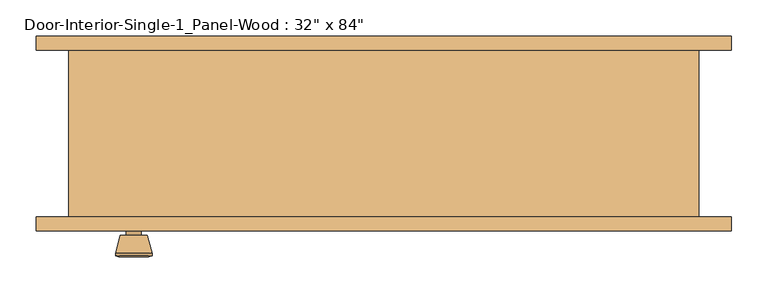
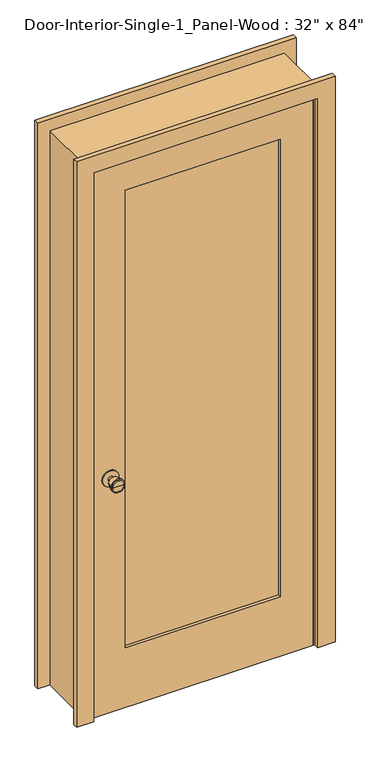
"""IFC4 building model written with IfcOpenShell, lengths in millimetres: door geometry."""

from ifc_helpers import new_model, si_unit, point, frame, frame_2d, origin, place, context, project, spatial, polyline, circle_curve, trimmed, segment, composite_curve, outline, extrude, faceted_brep, source, transform, mapped, element, save
from ifc_brep_helpers import plane_surface, cylinder_surface, revolved_surface, advanced_brep


def door_2631f38c(model_context):
    return source(origin(), model_context, "Body", "SolidModel", [
        advanced_brep(
        [(-342.9, -70.2, 914.4), (-352.9, -70.2, 914.4), (-332.9, -70.2, 914.4), (-322.4241324, -21.2, 914.4), (-363.3758676, -21.2, 914.4), (-342.9, -21.2, 914.4), (-317.9, -23.0278681, 914.4), (-367.9, -23.0278681, 914.4), (-317.9, -26.4915463, 914.4), (-367.9, -26.4915463, 914.4), (-324.263764, -51.2, 914.4), (-361.536236, -51.2, 914.4), (-332.9, -51.2, 914.4), (-352.9, -51.2, 914.4)],
        [
            (0, 1),
            (1, 2, circle_curve(frame((-342.9, -70.2, 914.4), z_axis=(0.0, -1.0, 0.0), x_axis=(-1.0, 0.0, 0.0)), 10.0)),
            (2, 0),
            (2, 1, circle_curve(frame((-342.9, -70.2, 914.4), z_axis=(0.0, -1.0, 0.0), x_axis=(-1.0, 0.0, 0.0)), 10.0)),
            (3, 4, circle_curve(frame((-342.9, -21.2, 914.4), z_axis=(0.0, 1.0, 0.0), x_axis=(-1.0, 0.0, 0.0)), 20.4758676)),
            (4, 5),
            (5, 3),
            (4, 3, circle_curve(frame((-342.9, -21.2, 914.4), z_axis=(0.0, 1.0, 0.0), x_axis=(-1.0, 0.0, 0.0)), 20.4758676)),
            (6, 7, circle_curve(frame((-342.9, -23.0278681, 914.4), z_axis=(0.0, 1.0, 0.0), x_axis=(-1.0, 0.0, 0.0)), 25.0)),
            (7, 4),
            (3, 6),
            (7, 6, circle_curve(frame((-342.9, -23.0278681, 914.4), z_axis=(0.0, 1.0, 0.0), x_axis=(-1.0, 0.0, 0.0)), 25.0)),
            (8, 9, circle_curve(frame((-342.9, -26.4915463, 914.4), z_axis=(0.0, 1.0, 0.0), x_axis=(-1.0, 0.0, 0.0)), 25.0)),
            (9, 7),
            (6, 8),
            (9, 8, circle_curve(frame((-342.9, -26.4915463, 914.4), z_axis=(0.0, 1.0, 0.0), x_axis=(-1.0, 0.0, 0.0)), 25.0)),
            (10, 11, circle_curve(frame((-342.9, -51.2, 914.4), z_axis=(0.0, 1.0, 0.0), x_axis=(-1.0, 0.0, 0.0)), 18.636236)),
            (11, 9),
            (8, 10),
            (11, 10, circle_curve(frame((-342.9, -51.2, 914.4), z_axis=(0.0, 1.0, 0.0), x_axis=(-1.0, 0.0, 0.0)), 18.636236)),
            (12, 13, circle_curve(frame((-342.9, -51.2, 914.4), z_axis=(0.0, 1.0, 0.0), x_axis=(-1.0, 0.0, 0.0)), 10.0)),
            (13, 11),
            (10, 12),
            (13, 12, circle_curve(frame((-342.9, -51.2, 914.4), z_axis=(0.0, 1.0, 0.0), x_axis=(-1.0, 0.0, 0.0)), 10.0)),
            (1, 13),
            (12, 2),
        ],
        [
            plane_surface(frame((-342.9, -70.2, 914.4), z_axis=(0.0, -1.0, 0.0), x_axis=(-1.0, 0.0, 0.0))),
            plane_surface(frame((-342.9, -21.2, 914.4), z_axis=(0.0, 1.0, 0.0), x_axis=(-1.0, 0.0, 0.0))),
            revolved_surface(polyline([(-363.3758676, -21.2, 914.4), (-367.9, -23.0278681, 914.4)]), (-342.9, -70.2, 914.4), (0.0, -1.0, 0.0)),
            cylinder_surface(frame((-342.9, -70.2, 914.4), z_axis=(0.0, -1.0, 0.0), x_axis=(-1.0, 0.0, 0.0)), 25.0),
            revolved_surface(polyline([(-367.9, -26.4915463, 914.4), (-361.536236, -51.2, 914.4)]), (-342.9, -70.2, 914.4), (0.0, -1.0, 0.0)),
            plane_surface(frame((-342.9, -51.2, 914.4), z_axis=(0.0, -1.0, 0.0), x_axis=(-1.0, 0.0, 0.0))),
            cylinder_surface(frame((-342.9, -70.2, 914.4), z_axis=(0.0, -1.0, 0.0), x_axis=(-1.0, 0.0, 0.0)), 10.0),
        ],
        [
            (0, [[1, 2, 3]]),
            (0, [[-3, 4, -1]]),
            (1, [[5, 6, 7]]),
            (1, [[8, -7, -6]]),
            (2, [[9, 10, -5, 11]]),
            (2, [[12, -11, -8, -10]]),
            (3, [[13, 14, -9, 15]]),
            (3, [[16, -15, -12, -14]]),
            (4, [[17, 18, -13, 19]]),
            (4, [[20, -19, -16, -18]]),
            (5, [[21, 22, -17, 23]]),
            (5, [[24, -23, -20, -22]]),
            (6, [[-2, 25, -21, 26]]),
            (6, [[-4, -26, -24, -25]]),
        ],
    ),
        extrude(outline(composite_curve([segment(trimmed(circle_curve(frame_2d((914.4, -342.9)), 30.0), [point((914.4, -372.9))], [point((914.4, -312.9))], False, "CARTESIAN"), True, "CONTINUOUS"), segment(trimmed(circle_curve(frame_2d((914.4, -342.9)), 30.0), [point((914.4, -312.9))], [point((914.4, -372.9))], False, "CARTESIAN"), True, "CONTINUOUS")], self_intersect=False)), frame((0.0, -76.2, 0.0), z_axis=(0.0, 1.0, 0.0), x_axis=(0.0, 0.0, 1.0)), (0.0, 0.0, 1.0), 6.0),
        advanced_brep(
        [(-342.9, -117.125, 914.4), (-332.9, -117.125, 914.4), (-352.9, -117.125, 914.4), (-322.4241324, -166.125, 914.4), (-342.9, -166.125, 914.4), (-363.3758676, -166.125, 914.4), (-317.9, -164.2971319, 914.4), (-367.9, -164.2971319, 914.4), (-317.9, -160.8334537, 914.4), (-367.9, -160.8334537, 914.4), (-324.263764, -136.125, 914.4), (-361.536236, -136.125, 914.4), (-332.9, -136.125, 914.4), (-352.9, -136.125, 914.4)],
        [
            (0, 1),
            (1, 2, circle_curve(frame((-342.9, -117.125, 914.4), z_axis=(0.0, 1.0, 0.0), x_axis=(-1.0, 0.0, 0.0)), 10.0)),
            (2, 0),
            (2, 1, circle_curve(frame((-342.9, -117.125, 914.4), z_axis=(0.0, 1.0, 0.0), x_axis=(-1.0, 0.0, 0.0)), 10.0)),
            (3, 4),
            (4, 5),
            (5, 3, circle_curve(frame((-342.9, -166.125, 914.4), z_axis=(0.0, -1.0, 0.0), x_axis=(-1.0, 0.0, 0.0)), 20.4758676)),
            (3, 5, circle_curve(frame((-342.9, -166.125, 914.4), z_axis=(0.0, -1.0, 0.0), x_axis=(-1.0, 0.0, 0.0)), 20.4758676)),
            (6, 3),
            (5, 7),
            (7, 6, circle_curve(frame((-342.9, -164.2971319, 914.4), z_axis=(0.0, -1.0, 0.0), x_axis=(-1.0, 0.0, 0.0)), 25.0)),
            (6, 7, circle_curve(frame((-342.9, -164.2971319, 914.4), z_axis=(0.0, -1.0, 0.0), x_axis=(-1.0, 0.0, 0.0)), 25.0)),
            (8, 6),
            (7, 9),
            (9, 8, circle_curve(frame((-342.9, -160.8334537, 914.4), z_axis=(0.0, -1.0, 0.0), x_axis=(-1.0, 0.0, 0.0)), 25.0)),
            (8, 9, circle_curve(frame((-342.9, -160.8334537, 914.4), z_axis=(0.0, -1.0, 0.0), x_axis=(-1.0, 0.0, 0.0)), 25.0)),
            (10, 8),
            (9, 11),
            (11, 10, circle_curve(frame((-342.9, -136.125, 914.4), z_axis=(0.0, -1.0, 0.0), x_axis=(-1.0, 0.0, 0.0)), 18.636236)),
            (10, 11, circle_curve(frame((-342.9, -136.125, 914.4), z_axis=(0.0, -1.0, 0.0), x_axis=(-1.0, 0.0, 0.0)), 18.636236)),
            (12, 10),
            (11, 13),
            (13, 12, circle_curve(frame((-342.9, -136.125, 914.4), z_axis=(0.0, -1.0, 0.0), x_axis=(-1.0, 0.0, 0.0)), 10.0)),
            (12, 13, circle_curve(frame((-342.9, -136.125, 914.4), z_axis=(0.0, -1.0, 0.0), x_axis=(-1.0, 0.0, 0.0)), 10.0)),
            (1, 12),
            (13, 2),
        ],
        [
            plane_surface(frame((-342.9, -117.125, 914.4), z_axis=(0.0, 1.0, 0.0), x_axis=(-1.0, 0.0, 0.0))),
            plane_surface(frame((-342.9, -166.125, 914.4), z_axis=(0.0, -1.0, 0.0), x_axis=(-1.0, 0.0, 0.0))),
            revolved_surface(polyline([(-363.3758676, -166.125, 914.4), (-367.9, -164.2971319, 914.4)]), (-342.9, -117.125, 914.4), (0.0, 1.0, 0.0)),
            cylinder_surface(frame((-342.9, -117.125, 914.4), z_axis=(0.0, 1.0, 0.0), x_axis=(-1.0, 0.0, 0.0)), 25.0),
            revolved_surface(polyline([(-367.9, -160.8334537, 914.4), (-361.536236, -136.125, 914.4)]), (-342.9, -117.125, 914.4), (0.0, 1.0, 0.0)),
            plane_surface(frame((-342.9, -136.125, 914.4), z_axis=(0.0, 1.0, 0.0), x_axis=(-1.0, 0.0, 0.0))),
            cylinder_surface(frame((-342.9, -117.125, 914.4), z_axis=(0.0, 1.0, 0.0), x_axis=(-1.0, 0.0, 0.0)), 10.0),
        ],
        [
            (0, [[1, 2, 3]]),
            (0, [[-3, 4, -1]]),
            (1, [[5, 6, 7]]),
            (1, [[-6, -5, 8]]),
            (2, [[9, -7, 10, 11]]),
            (2, [[-10, -8, -9, 12]]),
            (3, [[13, -11, 14, 15]]),
            (3, [[-14, -12, -13, 16]]),
            (4, [[17, -15, 18, 19]]),
            (4, [[-18, -16, -17, 20]]),
            (5, [[21, -19, 22, 23]]),
            (5, [[-22, -20, -21, 24]]),
            (6, [[25, -23, 26, -2]]),
            (6, [[-26, -24, -25, -4]]),
        ],
    ),
        extrude(outline(composite_curve([segment(trimmed(circle_curve(frame_2d((914.4, -342.9)), 30.0), [point((914.4, -372.9))], [point((914.4, -312.9))], False, "CARTESIAN"), True, "CONTINUOUS"), segment(trimmed(circle_curve(frame_2d((914.4, -342.9)), 30.0), [point((914.4, -312.9))], [point((914.4, -372.9))], False, "CARTESIAN"), True, "CONTINUOUS")], self_intersect=False)), frame((0.0, -117.125, 0.0), z_axis=(0.0, 1.0, 0.0), x_axis=(0.0, 0.0, 1.0)), (0.0, 0.0, 1.0), 6.0),
        faceted_brep([(431.8, -111.125, 0.0), (406.4, -111.125, 0.0), (406.4, -76.2, 0.0), (393.7, -76.2, 0.0), (393.7, -41.275, 0.0), (406.4, -41.275, 0.0), (406.4, 117.475, 0.0), (431.8, 117.475, 0.0), (431.8, 117.475, 2159.0), (431.8, -111.125, 2159.0), (406.4, 117.475, 2133.6), (-406.4, 117.475, 2133.6), (-406.4, 117.475, 0.0), (-431.8, 117.475, 0.0), (-431.8, 117.475, 2159.0), (406.4, -41.275, 2133.6), (393.7, -41.275, 2120.9), (-393.7, -41.275, 2120.9), (-393.7, -41.275, 0.0), (-406.4, -41.275, 0.0), (-406.4, -41.275, 2133.6), (393.7, -76.2, 2120.9), (406.4, -76.2, 2133.6), (-406.4, -76.2, 2133.6), (-406.4, -76.2, 0.0), (-393.7, -76.2, 0.0), (-393.7, -76.2, 2120.9), (406.4, -111.125, 2133.6), (-431.8, -111.125, 2159.0), (-431.8, -111.125, 0.0), (-406.4, -111.125, 0.0), (-406.4, -111.125, 2133.6)], [[[0, 1, 2, 3, 4, 5, 6, 7]], [[7, 8, 9, 0]], [[6, 10, 11, 12, 13, 14, 8, 7]], [[5, 15, 10, 6]], [[4, 16, 17, 18, 19, 20, 15, 5]], [[3, 21, 16, 4]], [[2, 22, 23, 24, 25, 26, 21, 3]], [[1, 27, 22, 2]], [[0, 9, 28, 29, 30, 31, 27, 1]], [[8, 14, 28, 9]], [[15, 20, 11, 10]], [[21, 26, 17, 16]], [[27, 31, 23, 22]], [[29, 13, 12, 19, 18, 25, 24, 30]], [[14, 13, 29, 28]], [[20, 19, 12, 11]], [[26, 25, 18, 17]], [[31, 30, 24, 23]]]),
        extrude(outline(polyline([(2133.6, -406.4), (0.0, -406.4), (0.0, 406.4), (2133.6, 406.4), (2133.6, -406.4)]), holes=[polyline([(2014.5375, -285.75), (2014.5375, 285.75), (231.775, 285.75), (231.775, -285.75), (2014.5375, -285.75)])]), frame((0.0, -111.125, 0.0), z_axis=(0.0, 1.0, 0.0), x_axis=(0.0, 0.0, 1.0)), (0.0, 0.0, 1.0), 34.925),
        extrude(outline(polyline([(285.75, -87.8416667), (285.75, -99.4833333), (-285.75, -99.4833333), (-285.75, -87.8416667), (285.75, -87.8416667)])), frame((0.0, 0.0, 231.775), z_axis=(0.0, 0.0, 1.0), x_axis=(1.0, 0.0, 0.0)), (0.0, 0.0, 1.0), 1782.7625),
        extrude(outline(polyline([(0.0, 476.25), (2203.45, 476.25), (2203.45, -476.25), (0.0, -476.25), (0.0, -412.75), (2139.95, -412.75), (2139.95, 412.75), (0.0, 412.75), (0.0, 476.25)])), frame((0.0, -130.175, 0.0), z_axis=(0.0, 1.0, 0.0), x_axis=(0.0, 0.0, 1.0)), (0.0, 0.0, 1.0), 19.05),
        extrude(outline(polyline([(0.0, 476.25), (2203.45, 476.25), (2203.45, -476.25), (0.0, -476.25), (0.0, -412.75), (2139.95, -412.75), (2139.95, 412.75), (0.0, 412.75), (0.0, 476.25)])), frame((0.0, 117.475, 0.0), z_axis=(0.0, 1.0, 0.0), x_axis=(0.0, 0.0, 1.0)), (0.0, 0.0, 1.0), 19.05),
    ])


if __name__ == "__main__":
    model = new_model("IFC4")
    model_context = context("Model", 3, world=origin())
    ifc_project = project(units=[si_unit("LENGTHUNIT", "METRE", prefix="MILLI")], contexts=[model_context])
    site = spatial("IfcSite", under=ifc_project)
    building = spatial("IfcBuilding", under=site)
    placement = place(None, origin())
    door_shape = door_2631f38c(model_context)
    element("IfcDoor", 1, ObjectType="Door-Interior-Single-1_Panel-Wood : 32\" x 84\"", at=placement, inside=building, context=model_context, shape_type="MappedRepresentation", body=[
        mapped(door_shape, transform((0.0, 0.0, 0.0), x_axis=(1.0, 0.0, 0.0), y_axis=(0.0, 1.0, 0.0), z_axis=(0.0, 0.0, 1.0))),
    ])
    save(model, "model.ifc")

# Revit data of these elements
# Type "Door-Interior-Single-1_Panel-Wood : 32\" x 84\""
#   Type Mark = "9"
#   Assembly Code = "C1020300"
#   Analytic Construction = "Wooden"
#   Top Rail = 0' - 4 11/16"
#   Thickness = 0' - 1 3/8"
#   Thermal Resistance (R) = 2.5876 (h·ft²·°F)/BTU
#   Swing Angle [instance default] = 90.00°
#   Stiles = 0' - 4 3/4"
#   Rough Width = 2' - 10"
#   Rough Height = 7' - 1"
#   Height = 7' - 0"
#   Width = 2' - 8"
#   Heat Transfer Coefficient (U) = 0.3865 BTU/(h·ft²·°F)
#   Bottom Rail = 0' - 9 1/8"
#   Trim Material = Cherry
#   Panel Material = Cherry
#   Frame Material = Cherry
#   Door Handle Material = Aluminum
#   Visual Light Transmittance = 0
#   Solar Heat Gain Coefficient = 0
#   Wall Closure = (empty or 0)
#   Function = (empty or 0)
# Element 1 (IfcDoor, "Door-Interior-Single-1_Panel-Wood : 32\" x 84\"")
#   Materials on its faces: "Cherry", "Aluminum"
# Materials
#   "Cherry": class "Wood", colour RGB 226 177 128, transparency 0, Description = "Prunus Serotina", Cost = 0
#   "Aluminum": class "Metal", colour RGB 247 247 247, transparency 0, Description = "Aluminum 6061", Cost = 0
